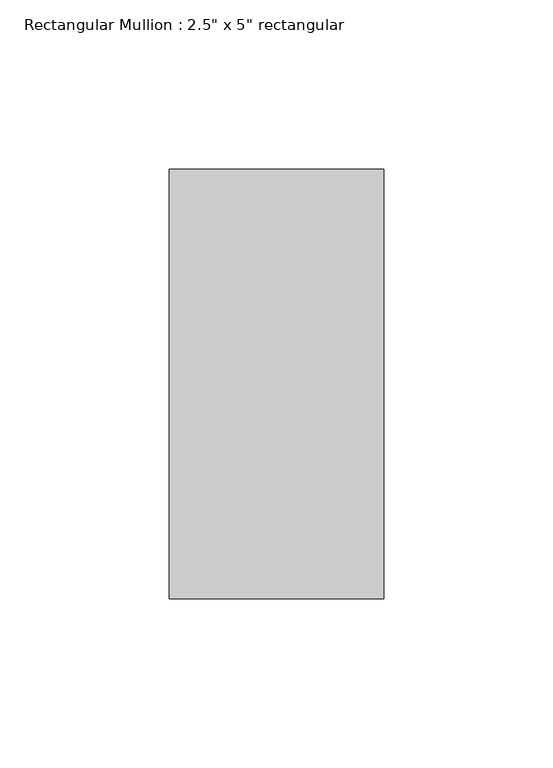
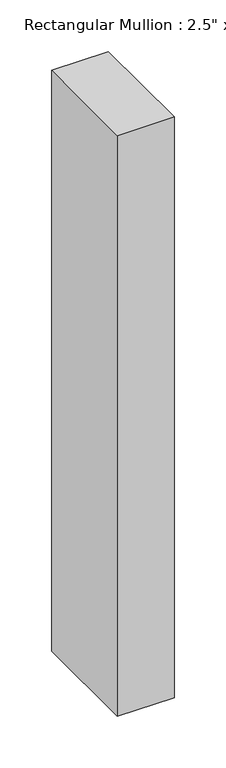
"""IFC4 building model written with IfcOpenShell, lengths in millimetres: member geometry."""

from ifc_helpers import new_model, si_unit, frame, origin, place, context, project, spatial, polyline, outline, extrude, source, transform, mapped, element, save


def member_27d1f1c9(model_context):
    return source(origin(), model_context, "Body", "SweptSolid", [
        extrude(outline(polyline([(31.75, 63.5), (31.75, -63.5), (-31.75, -63.5), (-31.75, 63.5), (31.75, 63.5)])), frame((0.0, 0.0, -685.9455358), z_axis=(0.0, 0.0, 1.0), x_axis=(1.0, 0.0, 0.0)), (0.0, 0.0, 1.0), 685.9455358),
    ])


if __name__ == "__main__":
    model = new_model("IFC4")
    model_context = context("Model", 3, world=origin())
    ifc_project = project(units=[si_unit("LENGTHUNIT", "METRE", prefix="MILLI")], contexts=[model_context])
    site = spatial("IfcSite", under=ifc_project)
    building = spatial("IfcBuilding", under=site)
    placement = place(None, origin())
    member_shape = member_27d1f1c9(model_context)
    element("IfcMember", 1, ObjectType="Rectangular Mullion : 2.5\" x 5\" rectangular", at=placement, inside=building, context=model_context, shape_type="MappedRepresentation", body=[
        mapped(member_shape, transform((0.0, 0.0, 0.0), x_axis=(1.0, 0.0, 0.0), y_axis=(0.0, 1.0, 0.0), z_axis=(0.0, 0.0, 1.0))),
    ])
    save(model, "model.ifc")

# Revit data of these elements
# Type "Rectangular Mullion : 2.5\" x 5\" rectangular"
#   built-in parameter 1007304 = 0.416667 (stored number, unit not read)
#   built-in parameter 1007301 = 0.104167 (stored number, unit not read)
#   built-in parameter 1007300 = 0.104167 (stored number, unit not read)
# Element 1 (IfcMember, "Rectangular Mullion : 2.5\" x 5\" rectangular")
#   Materials on its faces: "Aluminum"
# Materials
#   "Aluminum": class "Metal", colour RGB 247 247 247, transparency 0, Description = "Aluminum 6061", Cost = 0
